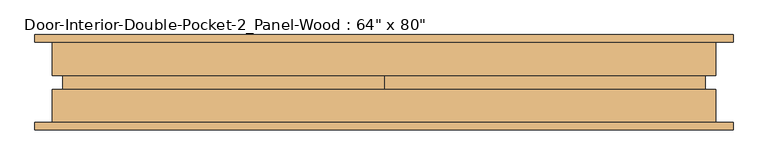
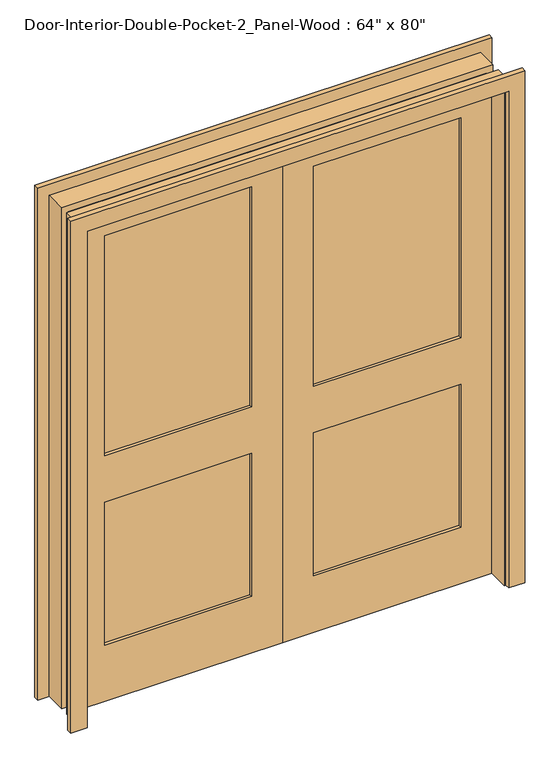
"""IFC4 building model written with IfcOpenShell, lengths in millimetres: door geometry."""

from ifc_helpers import new_model, si_unit, frame, origin, place, context, project, spatial, polyline, outline, extrude, source, transform, mapped, element, save


def door_18a53484(model_context):
    return source(origin(), model_context, "Body", "SweptSolid", [
        extrude(outline(polyline([(0.0, 819.15), (0.0, 882.65), (2101.85, 882.65), (2101.85, -882.65), (0.0, -882.65), (0.0, -819.15), (2038.35, -819.15), (2038.35, 819.15), (0.0, 819.15)])), frame((0.0, -120.65, 0.0), z_axis=(0.0, 1.0, 0.0), x_axis=(0.0, 0.0, 1.0)), (0.0, 0.0, 1.0), 19.05),
        extrude(outline(polyline([(0.0, 819.15), (0.0, 882.65), (2101.85, 882.65), (2101.85, -882.65), (0.0, -882.65), (0.0, -819.15), (2038.35, -819.15), (2038.35, 819.15), (0.0, 819.15)])), frame((0.0, 101.6, 0.0), z_axis=(0.0, 1.0, 0.0), x_axis=(0.0, 0.0, 1.0)), (0.0, 0.0, 1.0), 19.05),
        extrude(outline(polyline([(-120.65, -5.8208333), (-692.15, -5.8208333), (-692.15, 5.8208333), (-120.65, 5.8208333), (-120.65, -5.8208333)])), frame((0.0, 0.0, 1009.65), z_axis=(0.0, 0.0, 1.0), x_axis=(1.0, 0.0, 0.0)), (0.0, 0.0, 1.0), 903.2875),
        extrude(outline(polyline([(-120.65, -5.8208333), (-692.15, -5.8208333), (-692.15, 5.8208333), (-120.65, 5.8208333), (-120.65, -5.8208333)])), frame((0.0, 0.0, 231.775), z_axis=(0.0, 0.0, 1.0), x_axis=(1.0, 0.0, 0.0)), (0.0, 0.0, 1.0), 587.375),
        extrude(outline(polyline([(2032.0, -812.8), (0.0, -812.8), (0.0, 0.0), (2032.0, 0.0), (2032.0, -812.8)]), holes=[polyline([(1912.9375, -692.15), (1912.9375, -120.65), (1009.65, -120.65), (1009.65, -692.15), (1912.9375, -692.15)]), polyline([(819.15, -692.15), (819.15, -120.65), (231.775, -120.65), (231.775, -692.15), (819.15, -692.15)])]), frame((0.0, -17.4625, 0.0), z_axis=(0.0, 1.0, 0.0), x_axis=(0.0, 0.0, 1.0)), (0.0, 0.0, 1.0), 34.925),
        extrude(outline(polyline([(0.0, 838.2), (2057.4, 838.2), (2057.4, -838.2), (0.0, -838.2), (0.0, -812.8), (2032.0, -812.8), (2032.0, 812.8), (0.0, 812.8), (0.0, 838.2)])), frame((0.0, 17.4625, 0.0), z_axis=(0.0, 1.0, 0.0), x_axis=(0.0, 0.0, 1.0)), (0.0, 0.0, 1.0), 84.1375),
        extrude(outline(polyline([(0.0, 838.2), (2057.4, 838.2), (2057.4, -838.2), (0.0, -838.2), (0.0, -812.8), (2032.0, -812.8), (2032.0, 812.8), (0.0, 812.8), (0.0, 838.2)])), frame((0.0, -101.6, 0.0), z_axis=(0.0, 1.0, 0.0), x_axis=(0.0, 0.0, 1.0)), (0.0, 0.0, 1.0), 84.1375),
        extrude(outline(polyline([(692.15, -5.8208333), (120.65, -5.8208333), (120.65, 5.8208333), (692.15, 5.8208333), (692.15, -5.8208333)])), frame((0.0, 0.0, 1009.65), z_axis=(0.0, 0.0, 1.0), x_axis=(1.0, 0.0, 0.0)), (0.0, 0.0, 1.0), 903.2875),
        extrude(outline(polyline([(692.15, -5.8208333), (120.65, -5.8208333), (120.65, 5.8208333), (692.15, 5.8208333), (692.15, -5.8208333)])), frame((0.0, 0.0, 231.775), z_axis=(0.0, 0.0, 1.0), x_axis=(1.0, 0.0, 0.0)), (0.0, 0.0, 1.0), 587.375),
        extrude(outline(polyline([(2032.0, 0.0), (0.0, 0.0), (0.0, 812.8), (2032.0, 812.8), (2032.0, 0.0)]), holes=[polyline([(1912.9375, 120.65), (1912.9375, 692.15), (1009.65, 692.15), (1009.65, 120.65), (1912.9375, 120.65)]), polyline([(819.15, 120.65), (819.15, 692.15), (231.775, 692.15), (231.775, 120.65), (819.15, 120.65)])]), frame((0.0, -17.4625, 0.0), z_axis=(0.0, 1.0, 0.0), x_axis=(0.0, 0.0, 1.0)), (0.0, 0.0, 1.0), 34.925),
    ])


if __name__ == "__main__":
    model = new_model("IFC4")
    model_context = context("Model", 3, world=origin())
    ifc_project = project(units=[si_unit("LENGTHUNIT", "METRE", prefix="MILLI")], contexts=[model_context])
    site = spatial("IfcSite", under=ifc_project)
    building = spatial("IfcBuilding", under=site)
    placement = place(None, origin())
    door_shape = door_18a53484(model_context)
    element("IfcDoor", 1, ObjectType="Door-Interior-Double-Pocket-2_Panel-Wood : 64\" x 80\"", at=placement, inside=building, context=model_context, shape_type="MappedRepresentation", body=[
        mapped(door_shape, transform((0.0, 0.0, 0.0), x_axis=(1.0, 0.0, 0.0), y_axis=(0.0, 1.0, 0.0), z_axis=(0.0, 0.0, 1.0))),
    ])
    save(model, "model.ifc")

# Revit data of these elements
# Type "Door-Interior-Double-Pocket-2_Panel-Wood : 64\" x 80\""
#   Type Mark = "8"
#   Assembly Code = "C1020300"
#   Analytic Construction = "Wooden"
#   Top Rail = 0' - 4 11/16"
#   Thickness = 0' - 1 3/8"
#   Thermal Resistance (R) = 2.5876 (h·ft²·°F)/BTU
#   Stiles = 0' - 4 3/4"
#   Rough Width = 10' - 10"
#   Rough Height = 7' - 0 1/2"
#   Panel Width = 2' - 8"
#   Lock Rail = 0' - 7 1/2"
#   Location [instance default] = 2' - 9"
#   Height = 6' - 8"
#   Width = 5' - 4"
#   Heat Transfer Coefficient (U) = 0.3865 BTU/(h·ft²·°F)
#   Bottom Rail = 0' - 9 1/8"
#   Panel Open [instance default] = no
#   Trim Material = Cherry
#   Panel Material = Cherry
#   Frame Material = Cherry
#   Visual Light Transmittance = 0
#   Solar Heat Gain Coefficient = 0
#   Wall Closure = (empty or 0)
#   Function = (empty or 0)
# Element 1 (IfcDoor, "Door-Interior-Double-Pocket-2_Panel-Wood : 64\" x 80\"")
#   Materials on its faces: "Cherry"
# Materials
#   "Cherry": class "Wood", colour RGB 226 177 128, transparency 0, Description = "Prunus Serotina", Cost = 0
